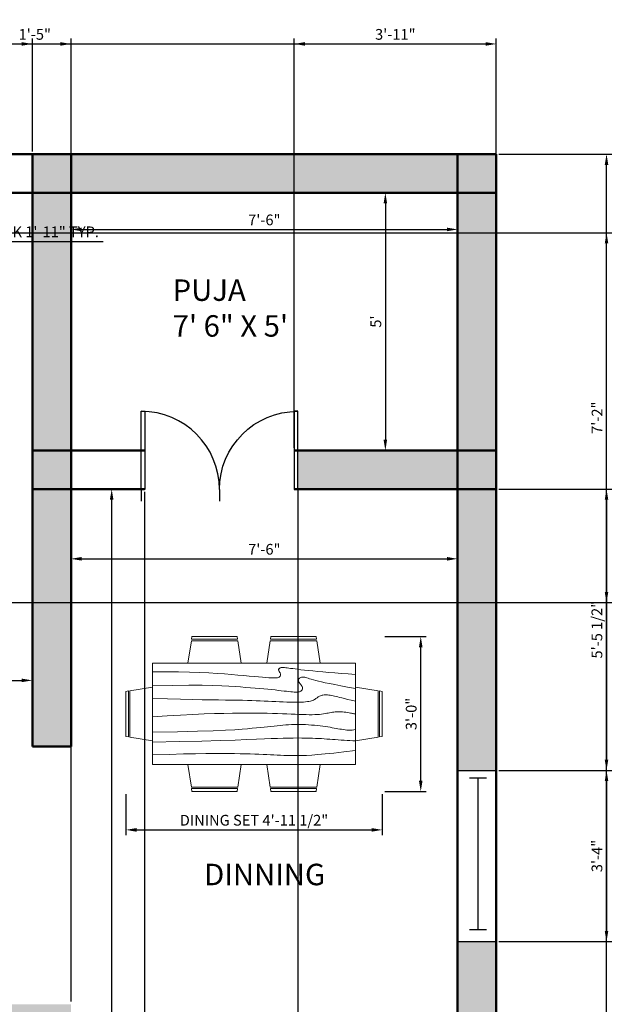
# Model space of a CAD drawing. Units: millimetres. Extents: x 2877 to 3173, y 802 to 1374.
# Tile 5 of 5: x 3035 to 3173, y 1144 to 1374. Entities that reach past the tile are written whole.
import ezdxf

# ---------------------------------------------------------------- set-up
doc = ezdxf.new("R2010")
doc.units = ezdxf.units.MM
for name, color, linetype, lineweight in [('A-AREA-IDEN', 150, 'Continuous', 25), ('A-WALL-PATT', 3, 'Continuous', 13), ('dimensions', 140, 'Continuous', 18), ('doors', 10, 'Continuous', 25), ('furniture', 70, 'Continuous', 18), ('walls', 50, 'Continuous', 50), ('windows', 190, 'Continuous', 25)]:
    doc.layers.add(name, color=color, linetype=linetype, lineweight=lineweight)
doc.styles.get("Standard").update_dxf_attribs({"font": 'arial.ttf'})
doc.dimstyles.new('ISO-25', dxfattribs={"dimtxt": 2.5, "dimasz": 2.5, "dimexe": 1.25, "dimexo": 0.625, "dimtad": 1, "dimdec": 0, "dimlunit": 3, "dimtxsty": 'Standard', "dimcen": 2.5, "dimadec": 0, "dimazin": 0, "dimtfac": 1, "dimtdec": 0, "dimtmove": 0, "dimatfit": 3, "dimfxl": 1, "dimarcsym": 0})

# ---------------------------------------------------------------- blocks, each defined once
blk = doc.blocks.new('*U2')
for p, q in [((0, 0), (0, -6)), ((40, 0), (40, -6))]:
    blk.add_line(p, q)
blk.add_lwpolyline([(0, 0), (0, 40), (1.75, 40), (1.75, 0)], close=True)
blk.add_arc((0, 0), 40, 0, 90)
blk = doc.blocks.new('*U4')
for p, q in [((0, 4), (0, 0)), ((36, 4), (36, 0)), ((0, 2), (36, 2))]:
    blk.add_line(p, q)
blk = doc.blocks.new('Dining Set - 36 x 72 in.')
for p, q in [((-22.2343, 26.00059), (-23.4847, 17.99762)), ((-22.2304, 26), (-5.7608, 26)), ((-22, 27.5), (-22.1562, 26.50042)), ((-5.8416, 26.5), (-22.1534, 26.5)), ((-22, 27.5), (-6, 27.5)), ((-5.8437, 26.49966), (-6, 27.5)), ((-4.5152, 17.99762), (-5.7655, 25.99926)), ((5.7657, 26.00059), (4.5153, 17.99762)), ((5.7696, 26), (22.2392, 26)), ((6, 27.5), (5.8438, 26.50042)), ((22.1584, 26.5), (5.8466, 26.5)), ((6, 27.5), (22, 27.5)), ((22.1563, 26.49966), (22, 27.5)), ((23.4848, 17.99762), (22.2345, 25.99926)), ((36, 18), (-36, 18)), ((-36, 18), (-36, -18)), ((36, -18), (36, 18)), ((-45.5, 8), (-44.5004, 8.15617)), ((-45.5, 8), (-45.5, -8)), ((-44.5, -8.15843), (-44.5, 8.15338)), ((-44.0006, 8.23428), (-35.9976, 9.48474)), ((-44, 8.23041), (-44, -8.23915)), ((44.0006, 8.23428), (35.9976, 9.48474)), ((44, 8.23041), (44, -8.23915)), ((44.5, -8.15843), (44.5, 8.15338)), ((45.5, 8), (44.5005, 8.15617)), ((45.5, 8), (45.5, -8)), ((-44.4997, -8.15631), (-45.5, -8)), ((-35.9976, -9.48476), (-43.9993, -8.2345)), ((35.9976, -9.48476), (43.9993, -8.2345)), ((44.4997, -8.15631), (45.5, -8)), ((-36, -18), (36, -18)), ((-22.2343, -26.0006), (-23.4847, -17.99762)), ((-4.5152, -17.99762), (-5.7655, -25.99928)), ((5.7657, -26.0006), (4.5153, -17.99762)), ((23.4848, -17.99762), (22.2345, -25.99928)), ((-22.2304, -26), (-5.7608, -26)), ((-22, -27.5), (-22.1562, -26.50044)), ((-5.8416, -26.5), (-22.1534, -26.5)), ((-22, -27.5), (-6, -27.5)), ((-5.8437, -26.49967), (-6, -27.5)), ((5.7696, -26), (22.2392, -26)), ((6, -27.5), (5.8438, -26.50044)), ((22.1584, -26.5), (5.8466, -26.5)), ((6, -27.5), (22, -27.5)), ((22.1563, -26.49967), (22, -27.5))]:
    blk.add_line(p, q)
for points in [[(-36, 15), (-31.1772, 14.97754), (-26.8079, 14.91406), (-22.8538, 14.81543), (-19.276, 14.6875), (-16.0362, 14.53613), (-13.0957, 14.36718), (-10.4159, 14.18652), (-7.9583, 14), (-5.6904, 13.81315), (-3.6035, 13.63021), (-1.6954, 13.45508), (0.0365, 13.29166), (1.5945, 13.14388), (2.9811, 13.01562), (4.1988, 12.9108), (5.25, 12.83333), (6.1393, 12.78613), (6.8802, 12.76823), (7.4883, 12.77767), (7.9792, 12.8125), (8.3685, 12.87077), (8.6719, 12.95052), (8.9049, 13.0498), (9.0833, 13.16666), (9.2205, 13.29899), (9.3216, 13.44401), (9.3895, 13.59879), (9.4271, 13.76041), (9.4373, 13.92594), (9.4232, 14.09245), (9.3875, 14.257), (9.3333, 14.41666), (9.2638, 14.56917), (9.1836, 14.71484), (9.0975, 14.85465), (9.0104, 14.98958), (8.9272, 15.1206), (8.8529, 15.2487), (8.7922, 15.37483), (8.75, 15.5), (8.7305, 15.62467), (8.7344, 15.74739), (8.7617, 15.86621), (8.8125, 15.97916), (8.8867, 16.08431), (8.9844, 16.17968), (9.1055, 16.26334), (9.25, 16.33333), (9.4189, 16.38802), (9.6172, 16.42708), (9.8506, 16.45052), (10.125, 16.45833), (10.4463, 16.45052), (10.8203, 16.42708), (11.2529, 16.38802), (11.75, 16.33333), (12.3184, 16.26318), (12.9694, 16.17838), (13.7151, 16.07991), (14.5677, 15.96875), (15.5395, 15.84586), (16.6426, 15.71224), (17.8893, 15.56884), (19.2917, 15.41666), (20.859, 15.25667), (22.5879, 15.08984), (24.4721, 14.91715), (26.5052, 14.73958), (28.6809, 14.5581), (30.9929, 14.3737), (33.4347, 14.18733), (36, 14)], [(-36, 10), (-28.9766, 10.14274), (-23.1725, 10.20442), (-18.4241, 10.19775), (-14.5677, 10.13541), (-11.4399, 10.03011), (-8.877, 9.89453), (-6.7154, 9.74137), (-4.7917, 9.58333), (-2.9698, 9.43082), (-1.2246, 9.28515), (0.4415, 9.14534), (2.026, 9.01041), (3.5266, 8.87939), (4.9408, 8.7513), (6.266, 8.62516), (7.5, 8.5), (8.6411, 8.37549), (9.6914, 8.2539), (10.6538, 8.13818), (11.5312, 8.03125), (12.3267, 7.93603), (13.043, 7.85547), (13.6831, 7.79248), (14.25, 7.75), (14.7471, 7.7303), (15.1797, 7.73307), (15.5537, 7.75732), (15.875, 7.80208), (16.1494, 7.86637), (16.3828, 7.94922), (16.5811, 8.04964), (16.75, 8.16666), (16.8944, 8.29915), (17.0143, 8.44531), (17.1089, 8.60319), (17.1771, 8.77083), (17.218, 8.94629), (17.2305, 9.1276), (17.2137, 9.31282), (17.1667, 9.5), (17.0895, 9.6875), (16.987, 9.875), (16.8649, 10.0625), (16.7292, 10.25), (16.5856, 10.4375), (16.4401, 10.625), (16.2985, 10.8125), (16.1667, 11), (16.05, 11.18733), (15.9518, 11.3737), (15.8752, 11.5581), (15.8229, 11.73958), (15.798, 11.91715), (15.8034, 12.08984), (15.842, 12.25667), (15.9167, 12.41666), (16.0295, 12.56836), (16.1784, 12.70833), (16.3605, 12.83268), (16.5729, 12.9375), (16.8127, 13.01888), (17.0768, 13.07291), (17.3625, 13.0957), (17.6667, 13.08333), (17.9894, 13.03312), (18.3418, 12.94726), (18.7382, 12.82918), (19.1927, 12.68229), (19.7195, 12.51001), (20.3327, 12.31575), (21.0465, 12.10294), (21.875, 11.875), (22.8357, 11.63354), (23.959, 11.37304), (25.2786, 11.08618), (26.8282, 10.76562), (28.6414, 10.40405), (30.752, 9.99414), (33.1936, 9.52856), (36, 9)], [(-36, 5.5), (-30.7157, 5.3348), (-26.069, 5.20963), (-21.9946, 5.11767), (-18.4271, 5.05208), (-15.3009, 5.00602), (-12.5508, 4.97265), (-10.1112, 4.94515), (-7.9167, 4.91666), (-5.909, 4.88167), (-4.0586, 4.83984), (-2.3429, 4.79215), (-0.7396, 4.73958), (0.7739, 4.6831), (2.22, 4.6237), (3.6213, 4.56233), (5, 4.5), (6.373, 4.43782), (7.7344, 4.3776), (9.0723, 4.32129), (10.375, 4.27083), (11.6309, 4.22819), (12.8281, 4.19531), (13.9551, 4.17415), (15, 4.16666), (15.954, 4.17448), (16.819, 4.19791), (17.6001, 4.23698), (18.3021, 4.29166), (18.9299, 4.36198), (19.4883, 4.44791), (19.9823, 4.54948), (20.4167, 4.66666), (20.7969, 4.79899), (21.1302, 4.94401), (21.4245, 5.09879), (21.6875, 5.26041), (21.9271, 5.42594), (22.1511, 5.59245), (22.3672, 5.757), (22.5834, 5.91666), (22.8065, 6.06868), (23.0404, 6.21093), (23.2879, 6.34147), (23.5521, 6.45833), (23.8358, 6.55957), (24.142, 6.64323), (24.4735, 6.70735), (24.8334, 6.75), (25.2235, 6.76969), (25.642, 6.76692), (26.0858, 6.74267), (26.5521, 6.69791), (27.0379, 6.63362), (27.5404, 6.55078), (28.0565, 6.45036), (28.5834, 6.33333), (29.1242, 6.19987), (29.7071, 6.04687), (30.3661, 5.87044), (31.1354, 5.66666), (32.0493, 5.43164), (33.142, 5.16146), (34.4475, 4.85221), (36, 4.5)], [(-36, -1), (-30.7915, -0.6591), (-26.0195, -0.38216), (-21.6519, -0.16284), (-17.6563, 0.00521), (-14.0005, 0.12833), (-10.6523, 0.21289), (-7.5796, 0.26522), (-4.75, 0.29166), (-2.134, 0.29793), (0.2878, 0.28711), (2.5317, 0.26163), (4.6146, 0.22396), (6.5529, 0.17651), (8.3633, 0.12174), (10.0623, 0.06209), (11.6667, 0), (13.1899, -0.06201), (14.6341, -0.1211), (15.9982, -0.17432), (17.2813, -0.21875), (18.4823, -0.25147), (19.6003, -0.26953), (20.6343, -0.27002), (21.5834, -0.25), (22.4481, -0.20768), (23.2357, -0.14584), (23.9549, -0.06836), (24.6146, 0.02083), (25.2235, 0.11784), (25.7904, 0.21875), (26.3241, 0.31966), (26.8334, 0.41666), (27.3265, 0.50618), (27.8099, 0.58593), (28.2894, 0.65397), (28.7709, 0.70833), (29.2601, 0.74707), (29.763, 0.76823), (30.2855, 0.76985), (30.8334, 0.75), (31.4088, 0.70784), (31.9994, 0.64713), (32.589, 0.57275), (33.1615, 0.48958), (33.7008, 0.4025), (34.1908, 0.3164), (34.6153, 0.23616), (34.9584, 0.16666), (35.2099, 0.11165), (35.3848, 0.07031), (35.504, 0.04069), (35.5886, 0.02083), (35.6594, 0.00879), (35.7377, 0.0026), (35.8442, 0.00032), (36, 0)], [(-36, -6.5), (-27.1843, -6.31267), (-20.084, -6.1263), (-14.469, -5.9419), (-10.1094, -5.76042), (-6.7752, -5.58285), (-4.2363, -5.41016), (-2.2629, -5.24333), (-0.625, -5.08334), (0.8708, -4.93099), (2.2715, -4.78646), (3.5872, -4.64974), (4.8281, -4.52084), (6.0046, -4.39974), (7.127, -4.28646), (8.2053, -4.18099), (9.25, -4.08334), (10.2705, -3.99382), (11.2734, -3.91407), (12.2647, -3.84603), (13.25, -3.79167), (14.2354, -3.75293), (15.2266, -3.73177), (16.2295, -3.73015), (17.25, -3.75), (18.2912, -3.79248), (19.3451, -3.85547), (20.4009, -3.93604), (21.4479, -4.03125), (22.4754, -4.13819), (23.4727, -4.25391), (24.4289, -4.37549), (25.3334, -4.5), (26.1785, -4.62492), (26.9694, -4.74935), (27.7145, -4.87281), (28.4219, -4.99479), (29.1, -5.11483), (29.7572, -5.23242), (30.4016, -5.34709), (31.0417, -5.45834), (31.6837, -5.56437), (32.3262, -5.65821), (32.9658, -5.73153), (33.599, -5.77604), (34.2224, -5.78345), (34.8327, -5.74545), (35.4264, -5.65373), (36, -5.5)], [(-36, -10), (-26.4022, -9.81299), (-18.4675, -9.62891), (-11.9839, -9.45069), (-6.7396, -9.28125), (-2.5226, -9.12354), (0.8789, -8.98047), (3.6769, -8.85498), (6.0833, -8.75), (8.2767, -8.66765), (10.3021, -8.60677), (12.1712, -8.56543), (13.8958, -8.54167), (15.4876, -8.53353), (16.9583, -8.53907), (18.3197, -8.55632), (19.5834, -8.58334), (20.7616, -8.61841), (21.8685, -8.66081), (22.9188, -8.71004), (23.9271, -8.76563), (24.9081, -8.82707), (25.8763, -8.89388), (26.8465, -8.96558), (27.8334, -9.04167), (28.8474, -9.12118), (29.8828, -9.20117), (30.93, -9.27824), (31.9792, -9.34896), (33.0205, -9.40991), (34.0443, -9.45768), (35.0407, -9.48885), (36, -9.5)], [(-36, -14.5), (-30.0881, -14.33513), (-25.0332, -14.21224), (-20.7312, -14.12647), (-17.0781, -14.07292), (-13.97, -14.04671), (-11.3027, -14.04297), (-8.9724, -14.05681), (-6.875, -14.08334), (-4.9224, -14.11833), (-3.0905, -14.16016), (-1.3709, -14.20785), (0.2448, -14.26042), (1.7647, -14.3169), (3.1973, -14.3763), (4.5507, -14.43767), (5.8333, -14.5), (7.0554, -14.5621), (8.235, -14.62175), (9.3922, -14.67652), (10.5469, -14.72396), (11.7192, -14.76164), (12.929, -14.78711), (14.1965, -14.79794), (15.5417, -14.79167), (16.9933, -14.76424), (18.6152, -14.70508), (20.4804, -14.60197), (22.6615, -14.44271), (25.2312, -14.21509), (28.2624, -13.9069), (31.8277, -13.50594), (36, -13)]]:
    blk.add_lwpolyline(points)
blk = doc.blocks.new('*D10')
at = {"layer": 'Defpoints', "color": 0, "transparency": 16777216}
for p in [(3037.62, 1219.71), (2917.62, 1213.28), (3037.62, 1213.28)]:
    blk.add_point(p, dxfattribs=at)
at = {"layer": 'dimensions', "color": 0, "lineweight": -2, "transparency": 16777216}
for p, q in [((2917.62, 1213.9), (2917.62, 1220.96)), ((3037.62, 1213.9), (3037.62, 1220.96)), ((2920.12, 1219.71), (3035.12, 1219.71))]:
    blk.add_line(p, q, dxfattribs=at)
at = {"layer": 'dimensions', "color": 0, "transparency": 16777216}
for points in [[(2920.12, 1220.13), (2920.12, 1219.3), (2917.62, 1219.71)], [(3035.12, 1220.13), (3035.12, 1219.3), (3037.62, 1219.71)]]:
    blk.add_solid(points, dxfattribs=at)
at = {"layer": 'dimensions', "color": 0, "transparency": 16777216, "insert": (2977.62, 1221.62), "char_height": 2.5, "attachment_point": 5}
blk.add_mtext("10'", dxfattribs=at)
blk = doc.blocks.new('*D12')
at = {"layer": 'Defpoints', "color": 0, "transparency": 16777216}
for p in [(3046.62, 1324.74), (3136.62, 1324.74), (3136.62, 1324.74)]:
    blk.add_point(p, dxfattribs=at)
at = {"layer": 'dimensions', "color": 0, "lineweight": -2, "transparency": 16777216}
for p, q in [((3046.62, 1325.37), (3046.62, 1325.99)), ((3136.62, 1325.37), (3136.62, 1325.99)), ((3049.12, 1324.74), (3134.12, 1324.74))]:
    blk.add_line(p, q, dxfattribs=at)
at = {"layer": 'dimensions', "color": 0, "transparency": 16777216}
for points in [[(3049.12, 1325.16), (3049.12, 1324.32), (3046.62, 1324.74)], [(3134.12, 1325.16), (3134.12, 1324.32), (3136.62, 1324.74)]]:
    blk.add_solid(points, dxfattribs=at)
at = {"layer": 'dimensions', "color": 0, "transparency": 16777216, "insert": (3091.62, 1326.64), "char_height": 2.5, "attachment_point": 5}
blk.add_mtext('7\'-6"', dxfattribs=at)
blk = doc.blocks.new('*D13')
at = {"layer": 'Defpoints', "color": 0, "transparency": 16777216}
for p in [(3123.12, 1333.28), (3119.8, 1273.28), (3123.12, 1273.28)]:
    blk.add_point(p, dxfattribs=at)
at = {"layer": 'dimensions', "color": 0, "lineweight": -2, "transparency": 16777216}
for p, q in [((3122.5, 1333.28), (3118.55, 1333.28)), ((3119.8, 1330.78), (3119.8, 1275.78)), ((3122.5, 1273.28), (3118.55, 1273.28))]:
    blk.add_line(p, q, dxfattribs=at)
at = {"layer": 'dimensions', "color": 0, "transparency": 16777216}
for points in [[(3119.38, 1330.78), (3120.21, 1330.78), (3119.8, 1333.28)], [(3119.38, 1275.78), (3120.21, 1275.78), (3119.8, 1273.28)]]:
    blk.add_solid(points, dxfattribs=at)
at = {"layer": 'dimensions', "color": 0, "transparency": 16777216, "insert": (3117.9, 1303.28), "char_height": 2.5, "attachment_point": 5, "rotation": 90}
blk.add_mtext("5'", dxfattribs=at)
blk = doc.blocks.new('*D14')
at = {"layer": 'Defpoints', "color": 0, "transparency": 16777216}
for p in [(3046.62, 1251.69), (3136.62, 1251.69), (3136.62, 1248.03)]:
    blk.add_point(p, dxfattribs=at)
at = {"layer": 'dimensions', "color": 0, "lineweight": -2, "transparency": 16777216}
for p, q in [((3046.62, 1251.06), (3046.62, 1246.78)), ((3136.62, 1251.06), (3136.62, 1246.78)), ((3049.12, 1248.03), (3134.12, 1248.03))]:
    blk.add_line(p, q, dxfattribs=at)
at = {"layer": 'dimensions', "color": 0, "transparency": 16777216}
for points in [[(3049.12, 1248.45), (3049.12, 1247.61), (3046.62, 1248.03)], [(3134.12, 1248.45), (3134.12, 1247.61), (3136.62, 1248.03)]]:
    blk.add_solid(points, dxfattribs=at)
at = {"layer": 'dimensions', "color": 0, "transparency": 16777216, "insert": (3091.62, 1249.93), "char_height": 2.5, "attachment_point": 5}
blk.add_mtext('7\'-6"', dxfattribs=at)
blk = doc.blocks.new('*D15')
at = {"layer": 'Defpoints', "color": 0, "transparency": 16777216}
for p in [(3056.09, 1264.28), (3061, 1264.28), (3061, 1012.28)]:
    blk.add_point(p, dxfattribs=at)
at = {"layer": 'dimensions', "color": 0, "lineweight": -2, "transparency": 16777216}
for p, q in [((3060.38, 1264.28), (3054.84, 1264.28)), ((3056.09, 1014.78), (3056.09, 1261.78)), ((3060.38, 1012.28), (3054.84, 1012.28))]:
    blk.add_line(p, q, dxfattribs=at)
at = {"layer": 'dimensions', "color": 0, "transparency": 16777216}
for points in [[(3055.67, 1261.78), (3056.5, 1261.78), (3056.09, 1264.28)], [(3055.67, 1014.78), (3056.5, 1014.78), (3056.09, 1012.28)]]:
    blk.add_solid(points, dxfattribs=at)
at = {"layer": 'dimensions', "color": 0, "transparency": 16777216, "insert": (3054.21, 1138.28), "char_height": 2.5, "attachment_point": 5, "rotation": 90}
blk.add_mtext("21'", dxfattribs=at)
blk = doc.blocks.new('*D24')
at = {"layer": 'Defpoints', "color": 0, "transparency": 16777216}
for p in [(3024.04, 1321.93), (3001.16, 1318.5), (3024.04, 1318.5)]:
    blk.add_point(p, dxfattribs=at)
at = {"layer": 'dimensions', "color": 0, "lineweight": -2, "transparency": 16777216}
for p, q in [((3001.16, 1319.12), (3001.16, 1323.18)), ((3024.04, 1319.12), (3024.04, 1323.18)), ((3003.66, 1321.93), (3021.54, 1321.93)), ((3024.04, 1321.93), (3054.08, 1321.93))]:
    blk.add_line(p, q, dxfattribs=at)
at = {"layer": 'dimensions', "color": 0, "transparency": 16777216}
for points in [[(3003.66, 1322.35), (3003.66, 1321.51), (3001.16, 1321.93)], [(3021.54, 1322.35), (3021.54, 1321.51), (3024.04, 1321.93)]]:
    blk.add_solid(points, dxfattribs=at)
at = {"layer": 'dimensions', "color": 0, "transparency": 16777216, "insert": (3040.31, 1323.85), "char_height": 2.5, "attachment_point": 5}
blk.add_mtext('SINK 1\'-11" TYP.', dxfattribs=at)
blk = doc.blocks.new('*D32')
at = {"layer": 'Defpoints', "color": 0, "transparency": 16777216}
for p in [(3059.37, 1193.86), (3119.08, 1193.86), (3119.08, 1184.9)]:
    blk.add_point(p, dxfattribs=at)
at = {"layer": 'dimensions', "color": 0, "lineweight": -2, "transparency": 16777216}
for p, q in [((3059.37, 1193.23), (3059.37, 1183.65)), ((3119.08, 1193.23), (3119.08, 1183.65)), ((3061.87, 1184.9), (3116.58, 1184.9))]:
    blk.add_line(p, q, dxfattribs=at)
at = {"layer": 'dimensions', "color": 0, "transparency": 16777216}
for points in [[(3061.87, 1185.32), (3061.87, 1184.48), (3059.37, 1184.9)], [(3116.58, 1185.32), (3116.58, 1184.48), (3119.08, 1184.9)]]:
    blk.add_solid(points, dxfattribs=at)
at = {"layer": 'dimensions', "color": 0, "transparency": 16777216, "insert": (3089.22, 1186.82), "char_height": 2.5, "attachment_point": 5}
blk.add_mtext('DINING SET 4\'-11 1/2"', dxfattribs=at)
blk = doc.blocks.new('*D33')
at = {"layer": 'Defpoints', "color": 0, "transparency": 16777216}
for p in [(3119.08, 1229.95), (3128.04, 1229.95), (3119.08, 1193.86)]:
    blk.add_point(p, dxfattribs=at)
at = {"layer": 'dimensions', "color": 0, "lineweight": -2, "transparency": 16777216}
for p, q in [((3119.71, 1229.95), (3129.29, 1229.95)), ((3128.04, 1196.36), (3128.04, 1227.45)), ((3119.71, 1193.86), (3129.29, 1193.86))]:
    blk.add_line(p, q, dxfattribs=at)
at = {"layer": 'dimensions', "color": 0, "transparency": 16777216}
for points in [[(3127.62, 1227.45), (3128.45, 1227.45), (3128.04, 1229.95)], [(3127.62, 1196.36), (3128.45, 1196.36), (3128.04, 1193.86)]]:
    blk.add_solid(points, dxfattribs=at)
at = {"layer": 'dimensions', "color": 0, "transparency": 16777216, "insert": (3126.14, 1211.9), "char_height": 2.5, "attachment_point": 5, "rotation": 90}
blk.add_mtext('3\'-0"', dxfattribs=at)
blk = doc.blocks.new('*D34')
at = {"layer": 'Defpoints', "color": 0, "transparency": 16777216}
for p in [(3145.62, 1367.94), (2908.62, 1342.28), (3145.62, 1342.28)]:
    blk.add_point(p, dxfattribs=at)
at = {"layer": 'dimensions', "color": 0, "lineweight": -2, "transparency": 16777216}
for p, q in [((2908.62, 1342.9), (2908.62, 1369.19)), ((3145.62, 1342.9), (3145.62, 1369.19)), ((2911.12, 1367.94), (3143.12, 1367.94))]:
    blk.add_line(p, q, dxfattribs=at)
at = {"layer": 'dimensions', "color": 0, "transparency": 16777216}
for points in [[(2911.12, 1368.36), (2911.12, 1367.52), (2908.62, 1367.94)], [(3143.12, 1368.36), (3143.12, 1367.52), (3145.62, 1367.94)]]:
    blk.add_solid(points, dxfattribs=at)
at = {"layer": 'dimensions', "color": 0, "transparency": 16777216, "insert": (3027.12, 1369.84), "char_height": 2.5, "attachment_point": 5}
blk.add_mtext('19\'-9"', dxfattribs=at)
blk = doc.blocks.new('*D35')
at = {"layer": 'Defpoints', "color": 0, "transparency": 16777216}
for p in [(3145.62, 1342.28), (3171.28, 1342.28), (3145.62, 829.28)]:
    blk.add_point(p, dxfattribs=at)
at = {"layer": 'dimensions', "color": 0, "lineweight": -2, "transparency": 16777216}
for p, q in [((3146.25, 1342.28), (3172.53, 1342.28)), ((3171.28, 831.78), (3171.28, 1339.78)), ((3146.25, 829.28), (3172.53, 829.28))]:
    blk.add_line(p, q, dxfattribs=at)
at = {"layer": 'dimensions', "color": 0, "transparency": 16777216}
for points in [[(3170.87, 1339.78), (3171.7, 1339.78), (3171.28, 1342.28)], [(3170.87, 831.78), (3171.7, 831.78), (3171.28, 829.28)]]:
    blk.add_solid(points, dxfattribs=at)
at = {"layer": 'dimensions', "color": 0, "transparency": 16777216, "insert": (3169.38, 1085.78), "char_height": 2.5, "attachment_point": 5, "rotation": 90}
blk.add_mtext('42\'-9"', dxfattribs=at)
blk = doc.blocks.new('*D40')
at = {"layer": 'Defpoints', "color": 0, "transparency": 16777216}
for p in [(3063.76, 1264.28), (3099.39, 1264.17), (3099.39, 803.61)]:
    blk.add_point(p, dxfattribs=at)
at = {"layer": 'dimensions', "color": 0, "lineweight": -2, "transparency": 16777216}
for p, q in [((3063.76, 1263.65), (3063.76, 802.36)), ((3099.39, 1263.55), (3099.39, 802.36)), ((3066.26, 803.61), (3096.89, 803.61))]:
    blk.add_line(p, q, dxfattribs=at)
at = {"layer": 'dimensions', "color": 0, "transparency": 16777216}
for points in [[(3066.26, 804.03), (3066.26, 803.2), (3063.76, 803.61)], [(3096.89, 804.03), (3096.89, 803.2), (3099.39, 803.61)]]:
    blk.add_solid(points, dxfattribs=at)
at = {"layer": 'dimensions', "color": 0, "transparency": 16777216, "insert": (3081.57, 805.53), "char_height": 2.5, "attachment_point": 5}
blk.add_mtext('2\'-11 1/2"', dxfattribs=at)
blk = doc.blocks.new('*D41')
at = {"layer": 'Defpoints', "color": 0, "transparency": 16777216}
for p in [(3145.62, 1367.94), (3098.59, 1273.28), (3145.62, 1273.28)]:
    blk.add_point(p, dxfattribs=at)
at = {"layer": 'dimensions', "color": 0, "lineweight": -2, "transparency": 16777216}
for p, q in [((3098.59, 1273.9), (3098.59, 1369.19)), ((3145.62, 1273.9), (3145.62, 1369.19)), ((3101.09, 1367.94), (3143.12, 1367.94))]:
    blk.add_line(p, q, dxfattribs=at)
at = {"layer": 'dimensions', "color": 0, "transparency": 16777216}
for points in [[(3101.09, 1368.36), (3101.09, 1367.52), (3098.59, 1367.94)], [(3143.12, 1368.36), (3143.12, 1367.52), (3145.62, 1367.94)]]:
    blk.add_solid(points, dxfattribs=at)
at = {"layer": 'dimensions', "color": 0, "transparency": 16777216, "insert": (3122.11, 1369.84), "char_height": 2.5, "attachment_point": 5}
blk.add_mtext('3\'-11"', dxfattribs=at)
blk = doc.blocks.new('*D45')
at = {"layer": 'Defpoints', "color": 0, "transparency": 16777216}
for p in [(3029.69, 1323.97), (3171.28, 1323.97), (3029.69, 1237.82)]:
    blk.add_point(p, dxfattribs=at)
at = {"layer": 'dimensions', "color": 0, "lineweight": -2, "transparency": 16777216}
for p, q in [((3030.32, 1323.97), (3172.53, 1323.97)), ((3171.28, 1240.32), (3171.28, 1321.47)), ((3030.32, 1237.82), (3172.53, 1237.82))]:
    blk.add_line(p, q, dxfattribs=at)
at = {"layer": 'dimensions', "color": 0, "transparency": 16777216}
for points in [[(3170.87, 1321.47), (3171.7, 1321.47), (3171.28, 1323.97)], [(3170.87, 1240.32), (3171.7, 1240.32), (3171.28, 1237.82)]]:
    blk.add_solid(points, dxfattribs=at)
at = {"layer": 'dimensions', "color": 0, "transparency": 16777216, "insert": (3169.4, 1280.89), "char_height": 2.5, "attachment_point": 5, "rotation": 90}
blk.add_mtext('7\'-2"', dxfattribs=at)
blk = doc.blocks.new('*D49')
at = {"layer": 'Defpoints', "color": 0, "transparency": 16777216}
for p in [(3046.62, 1367.94), (3029.73, 1144.28), (3046.62, 1144.28)]:
    blk.add_point(p, dxfattribs=at)
at = {"layer": 'dimensions', "color": 0, "lineweight": -2, "transparency": 16777216}
for p, q in [((3029.73, 1144.9), (3029.73, 1369.19)), ((3046.62, 1144.9), (3046.62, 1369.19)), ((3032.23, 1367.94), (3044.12, 1367.94))]:
    blk.add_line(p, q, dxfattribs=at)
at = {"layer": 'dimensions', "color": 0, "transparency": 16777216}
for points in [[(3032.23, 1368.36), (3032.23, 1367.52), (3029.73, 1367.94)], [(3044.12, 1368.36), (3044.12, 1367.52), (3046.62, 1367.94)]]:
    blk.add_solid(points, dxfattribs=at)
at = {"layer": 'dimensions', "color": 0, "transparency": 16777216, "insert": (3038.18, 1369.84), "char_height": 2.5, "attachment_point": 5}
blk.add_mtext('1\'-5"', dxfattribs=at)
blk = doc.blocks.new('*D52')
at = {"layer": 'Defpoints', "color": 0, "transparency": 16777216}
for p in [(3037.62, 1367.94), (2993.21, 1342.28), (3037.62, 1342.28)]:
    blk.add_point(p, dxfattribs=at)
at = {"layer": 'dimensions', "color": 0, "lineweight": -2, "transparency": 16777216}
for p, q in [((2993.21, 1342.9), (2993.21, 1369.19)), ((3037.62, 1342.9), (3037.62, 1369.19)), ((2995.71, 1367.94), (3035.12, 1367.94))]:
    blk.add_line(p, q, dxfattribs=at)
at = {"layer": 'dimensions', "color": 0, "transparency": 16777216}
for points in [[(2995.71, 1368.36), (2995.71, 1367.52), (2993.21, 1367.94)], [(3035.12, 1368.36), (3035.12, 1367.52), (3037.62, 1367.94)]]:
    blk.add_solid(points, dxfattribs=at)
at = {"layer": 'dimensions', "color": 0, "transparency": 16777216, "insert": (3015.41, 1369.86), "char_height": 2.5, "attachment_point": 5}
blk.add_mtext('3\'-8 1/2"', dxfattribs=at)
blk = doc.blocks.new('*D60')
at = {"layer": 'Defpoints', "color": 0, "transparency": 16777216}
for p in [(3145.62, 1198.76), (3145.62, 1158.87), (3171.28, 1158.87)]:
    blk.add_point(p, dxfattribs=at)
at = {"layer": 'dimensions', "color": 0, "lineweight": -2, "transparency": 16777216}
for p, q in [((3146.25, 1198.76), (3172.53, 1198.76)), ((3171.28, 1196.26), (3171.28, 1161.37)), ((3146.25, 1158.87), (3172.53, 1158.87))]:
    blk.add_line(p, q, dxfattribs=at)
at = {"layer": 'dimensions', "color": 0, "transparency": 16777216}
for points in [[(3170.87, 1196.26), (3171.7, 1196.26), (3171.28, 1198.76)], [(3170.87, 1161.37), (3171.7, 1161.37), (3171.28, 1158.87)]]:
    blk.add_solid(points, dxfattribs=at)
at = {"layer": 'dimensions', "color": 0, "transparency": 16777216, "insert": (3169.38, 1178.82), "char_height": 2.5, "attachment_point": 5, "rotation": 90}
blk.add_mtext('3\'-4"', dxfattribs=at)
blk = doc.blocks.new('*D61')
at = {"layer": 'Defpoints', "color": 0, "transparency": 16777216}
for p in [(3145.62, 1264.28), (3145.62, 1198.76), (3171.28, 1198.76)]:
    blk.add_point(p, dxfattribs=at)
at = {"layer": 'dimensions', "color": 0, "lineweight": -2, "transparency": 16777216}
for p, q in [((3146.25, 1264.28), (3172.53, 1264.28)), ((3171.28, 1261.78), (3171.28, 1201.26)), ((3146.25, 1198.76), (3172.53, 1198.76))]:
    blk.add_line(p, q, dxfattribs=at)
at = {"layer": 'dimensions', "color": 0, "transparency": 16777216}
for points in [[(3170.87, 1261.78), (3171.7, 1261.78), (3171.28, 1264.28)], [(3170.87, 1201.26), (3171.7, 1201.26), (3171.28, 1198.76)]]:
    blk.add_solid(points, dxfattribs=at)
at = {"layer": 'dimensions', "color": 0, "transparency": 16777216, "insert": (3169.37, 1231.52), "char_height": 2.5, "attachment_point": 5, "rotation": 90}
blk.add_mtext('5\'-5 1/2"', dxfattribs=at)

msp = doc.modelspace()

# ---------------------------------------------------------------- hatches: boundary and pattern name
at = {"layer": 'A-WALL-PATT'}
h = msp.add_hatch(color=256, dxfattribs=at)
h.dxf.hatch_style = 1
h.paths.add_polyline_path([(3046.62, 1333.28), (3037.62, 1333.28), (3037.62, 1273.28), (3046.62, 1273.28)])
h.paths.add_polyline_path([(3046.62, 1273.28), (3037.62, 1273.28), (3037.62, 1264.28), (3046.62, 1264.28)])
h.paths.add_polyline_path([(3046.62, 1264.28), (3037.62, 1264.28), (3037.62, 1204.28), (3046.62, 1204.28)])
h.paths.add_polyline_path([(3136.62, 1273.28), (3099.39, 1273.28), (3099.39, 1264.28), (3136.62, 1264.28)])
h.paths.add_polyline_path([(3145.62, 1273.28), (3136.62, 1273.28), (3136.62, 1264.28), (3145.62, 1264.28)])
h.paths.add_polyline_path([(3145.62, 1264.28), (3136.62, 1264.28), (3136.62, 1198.76), (3145.62, 1198.76)])
h.paths.add_polyline_path([(3145.62, 1333.28), (3136.62, 1333.28), (3136.62, 1273.28), (3145.62, 1273.28)])
h.paths.add_polyline_path([(3145.62, 1342.28), (3136.62, 1342.28), (3136.62, 1333.28), (3145.62, 1333.28)])
h.paths.add_polyline_path([(3136.62, 1342.28), (3046.62, 1342.28), (3046.62, 1333.28), (3136.62, 1333.28)])
h.paths.add_polyline_path([(3046.62, 1342.28), (3037.62, 1342.28), (3037.62, 1333.28), (3046.62, 1333.28)])
h.paths.add_polyline_path([(2917.62, 1333.28), (2908.62, 1333.28), (2908.62, 1301.43), (2917.62, 1301.43)])
h.paths.add_polyline_path([(2917.62, 1257.52), (2908.62, 1257.52), (2908.62, 1213.28), (2917.62, 1213.28)])
h.paths.add_polyline_path([(2989.62, 1213.28), (2917.62, 1213.28), (2917.62, 1204.28), (2989.62, 1204.28)])
h.paths.add_polyline_path([(2998.62, 1213.28), (2989.62, 1213.28), (2989.62, 1204.28), (2998.62, 1204.28)])
h.paths.add_polyline_path([(2998.62, 1204.28), (2989.62, 1204.28), (2989.62, 1144.28), (2998.62, 1144.28)])
h.paths.add_polyline_path([(2998.62, 1144.28), (2989.62, 1144.28), (2989.62, 1135.28), (2998.62, 1135.28)])
h.paths.add_polyline_path([(2989.62, 1144.28), (2977.25, 1144.28), (2977.25, 1137.64), (2977.25, 1135.28), (2989.62, 1135.28)])
h.paths.add_polyline_path([(3006.77, 1141.79), (3006.77, 1144.28), (2998.62, 1144.28), (2998.62, 1135.28), (3007.71, 1135.28, -0.072018)])
h.paths.add_polyline_path([(3046.62, 1135.28), (3037.62, 1135.28), (3037.62, 1012.28), (3046.62, 1012.28)])
h.paths.add_polyline_path([(3046.62, 1144.28), (3037.62, 1144.28), (3037.62, 1135.28), (3046.62, 1135.28)])
h.paths.add_polyline_path([(3037.62, 1144.28), (3029.73, 1144.28), (3029.73, 1141.79), (3029.73, 1135.28), (3037.62, 1135.28)])
h.paths.add_polyline_path([(3145.62, 1158.87), (3136.62, 1158.87), (3136.62, 1012.28), (3145.62, 1012.28)])
h.paths.add_polyline_path([(3145.62, 1003.28), (3136.62, 1003.28), (3136.62, 838.28), (3145.62, 838.28)])
h.paths.add_polyline_path([(3145.62, 1012.28), (3136.62, 1012.28), (3136.62, 1003.28), (3145.62, 1003.28)])
h.paths.add_polyline_path([(3136.62, 1012.28), (3109.83, 1012.28), (3109.83, 1006.01), (3109.83, 1003.28), (3136.62, 1003.28)])
h.paths.add_polyline_path([(3073.41, 1012.28), (3046.62, 1012.28), (3046.62, 1003.28), (3073.41, 1003.28), (3073.41, 1006.01)])
h.paths.add_polyline_path([(3046.62, 1012.28), (3037.62, 1012.28), (3037.62, 1003.28), (3046.62, 1003.28)])
h.paths.add_polyline_path([(3046.62, 1003.28), (3037.62, 1003.28), (3037.62, 943.28), (3046.62, 943.28)])
h.paths.add_polyline_path([(3136.62, 838.28), (2917.62, 838.28), (2917.62, 829.28), (3136.62, 829.28)])
h.paths.add_polyline_path([(3145.62, 838.28), (3136.62, 838.28), (3136.62, 829.28), (3145.62, 829.28)])
h.paths.add_polyline_path([(2917.62, 934.28), (2908.62, 934.28), (2908.62, 838.28), (2917.62, 838.28)])
h.paths.add_polyline_path([(2917.62, 838.28), (2908.62, 838.28), (2908.62, 829.28), (2917.62, 829.28)])
h.paths.add_polyline_path([(2917.62, 943.28), (2908.62, 943.28), (2908.62, 934.28), (2917.62, 934.28)])
h.paths.add_polyline_path([(2966.07, 943.28), (2917.62, 943.28), (2917.62, 934.28), (2966.07, 934.28)])
h.paths.add_polyline_path([(3046.62, 943.28), (3037.62, 943.28), (3037.62, 934.28), (3046.62, 934.28)])
h.paths.add_polyline_path([(3037.62, 943.28), (3008.74, 943.28), (3008.74, 934.28), (3037.62, 934.28)])

# ---------------------------------------------------------------- linework, layer by layer
at = {"layer": 'walls'}
for p, q in [((2908.62, 1342.28), (3145.62, 1342.28)), ((3037.62, 1342.28), (3037.62, 1204.28)), ((3046.62, 1342.28), (3046.62, 1204.28)), ((3136.62, 1342.28), (3136.62, 829.28)), ((3145.62, 1342.28), (3145.62, 829.28)), ((2908.62, 1333.28), (3145.62, 1333.28)), ((3037.62, 1273.28), (3063.76, 1273.28)), ((3098.59, 1273.28), (3145.62, 1273.28)), ((3037.62, 1264.28), (3063.76, 1264.28)), ((3081.18, 1264.28), (3081.18, 1264.28)), ((3098.59, 1264.28), (3145.62, 1264.28)), ((3037.62, 1204.28), (3046.62, 1204.28))]:
    msp.add_line(p, q, dxfattribs=at)
at = {"layer": 'windows'}
for p, q in [((3136.62, 1198.76), (3145.62, 1198.76)), ((3136.62, 1158.87), (3145.62, 1158.87))]:
    msp.add_line(p, q, dxfattribs=at)

# ---------------------------------------------------------------- block references
at = {"layer": 'doors', "yscale": 0.4552510015893225, "zscale": 0.4552510015893225}
for p, xscale in [((3062.97, 1264.17), 0.4552510015893225), ((3099.39, 1264.17), -0.4552510015893225)]:
    msp.add_blockref('*U2', p, dxfattribs=dict(at, xscale=xscale))
at = {"layer": 'furniture', "xscale": 0.6562079688977632, "yscale": 0.6562079688977632, "zscale": 0.6562079688977632}
msp.add_blockref('Dining Set - 36 x 72 in.', (3089.22, 1211.9), dxfattribs=at)
at = {"layer": 'windows', "xscale": 0.9804508946843826, "yscale": 0.9804508946843826, "zscale": 0.9804508946843826, "rotation": 90}
msp.add_blockref('*U4', (3143.34, 1161.73), dxfattribs=at)

# ---------------------------------------------------------------- texts
at = {"layer": 'A-AREA-IDEN', "char_height": 5, "attachment_point": 1}
for s, width, insert in [('PUJA\\P7\' 6" X 5\'', 49.0592, (3070.28, 1313.1)), ('DINNING', 37.8063, (3077.61, 1177.01))]:
    msp.add_mtext_dynamic_manual_height_columns(s, width=width, gutter_width=12.5, heights=[0], dxfattribs=dict(at, insert=insert))

# ---------------------------------------------------------------- dimensions: what is measured, and where the dimension line sits
at = {"layer": 'dimensions'}
for base, p1, p2, override, picture, middle in [((3037.62, 1367.94), (2993.21, 1342.28), (3037.62, 1342.28), {"dimdec": 1, "dimlfac": 1, "dimrnd": 0, "dimzin": 1, "dimdsep": 46, "dimlunit": 4, "dimfrac": 2}, '*D52', (3015.41, 1369.86)), ((3145.62, 1367.94), (2908.62, 1342.28), (3145.62, 1342.28), {"dimdec": 1, "dimlfac": 1, "dimrnd": 0, "dimzin": 1, "dimdsep": 46, "dimlunit": 4, "dimfrac": 2}, '*D34', (3027.12, 1369.84)), ((3046.62, 1367.94), (3029.73, 1144.28), (3046.62, 1144.28), {"dimdec": 1, "dimlfac": 1, "dimrnd": 0, "dimzin": 1, "dimdsep": 46, "dimlunit": 4, "dimfrac": 2}, '*D49', (3038.18, 1369.84)), ((3145.62, 1367.94), (3098.59, 1273.28), (3145.62, 1273.28), {"dimdec": 1, "dimlfac": 1, "dimrnd": 0, "dimzin": 1, "dimdsep": 46, "dimlunit": 4, "dimfrac": 2}, '*D41', (3122.11, 1369.84)), ((3136.62, 1324.74), (3046.62, 1324.74), (3136.62, 1324.74), {"dimclrd": 0, "dimclre": 0, "dimclrt": 0}, '*D12', (3091.62, 1326.64)), ((3099.39, 803.61), (3063.76, 1264.28), (3099.39, 1264.17), {"dimdec": 1, "dimlfac": 1, "dimrnd": 0, "dimzin": 1, "dimdsep": 46, "dimlunit": 4, "dimfrac": 2}, '*D40', (3081.57, 805.53)), ((3136.62, 1248.03), (3046.62, 1251.69), (3136.62, 1251.69), {"dimclrd": 0, "dimclre": 0, "dimclrt": 0}, '*D14', (3091.62, 1249.93)), ((3037.62, 1219.71), (2917.62, 1213.28), (3037.62, 1213.28), {"dimclrd": 0, "dimclre": 0, "dimclrt": 0}, '*D10', (2977.62, 1221.62))]:
    dim = msp.add_linear_dim(base=base, p1=p1, p2=p2, dimstyle='ISO-25', override=override, dxfattribs=at)
    dim.commit()
    dim.dimension.update_dxf_attribs({"geometry": picture, "text_midpoint": middle})
for base, p1, p2, override, picture, middle in [((3171.28, 1342.28), (3145.62, 829.28), (3145.62, 1342.28), {"dimdec": 1, "dimlfac": 1, "dimrnd": 0, "dimzin": 1, "dimdsep": 46, "dimlunit": 4, "dimfrac": 2}, '*D35', (3169.38, 1085.78)), ((3119.8, 1273.28), (3123.12, 1333.28), (3123.12, 1273.28), {"dimclrd": 0, "dimclre": 0, "dimclrt": 0}, '*D13', (3117.9, 1303.28)), ((3171.2848, 1323.9689), (3029.6924, 1237.8157), (3029.6924, 1323.9689), {"dimdec": 1, "dimlfac": 1, "dimrnd": 0, "dimzin": 1, "dimdsep": 46, "dimlunit": 4, "dimfrac": 2}, '*D45', (3169.4047, 1280.8923)), ((3056.09, 1264.28), (3061, 1012.28), (3061, 1264.28), {"dimclrd": 0, "dimclre": 0, "dimclrt": 0}, '*D15', (3054.21, 1138.28)), ((3171.28, 1198.76), (3145.62, 1264.28), (3145.62, 1198.76), {"dimdec": 1, "dimlfac": 1, "dimrnd": 0, "dimzin": 1, "dimdsep": 46, "dimlunit": 4, "dimfrac": 2}, '*D61', (3169.37, 1231.52)), ((3128.04, 1229.95), (3119.08, 1193.86), (3119.08, 1229.95), {"dimdec": 1, "dimlfac": 1, "dimrnd": 0, "dimzin": 1, "dimdsep": 46, "dimlunit": 4, "dimfrac": 2}, '*D33', (3126.14, 1211.9)), ((3171.28, 1158.87), (3145.62, 1198.76), (3145.62, 1158.87), {"dimdec": 1, "dimlfac": 1, "dimrnd": 0, "dimzin": 1, "dimdsep": 46, "dimlunit": 4, "dimfrac": 2}, '*D60', (3169.38, 1178.82))]:
    dim = msp.add_linear_dim(base=base, p1=p1, p2=p2, angle=90, dimstyle='ISO-25', override=override, dxfattribs=at)
    dim.commit()
    dim.dimension.update_dxf_attribs({"geometry": picture, "text_midpoint": middle})
for base, p1, p2, text, picture, middle in [((3024.04, 1321.93), (3001.16, 1318.5), (3024.04, 1318.5), 'SINK <> TYP.', '*D24', (3040.31, 1323.85)), ((3119.08, 1184.9), (3059.37, 1193.86), (3119.08, 1193.86), 'DINING SET <>', '*D32', (3089.22, 1186.82))]:
    dim = msp.add_linear_dim(base=base, p1=p1, p2=p2, text=text, dimstyle='ISO-25', override={"dimdec": 1, "dimlfac": 1, "dimrnd": 0, "dimzin": 1, "dimdsep": 46, "dimlunit": 4, "dimfrac": 2}, dxfattribs=at)
    dim.commit()
    dim.dimension.update_dxf_attribs({"geometry": picture, "text_midpoint": middle})

doc.saveas('drawing.dxf')
